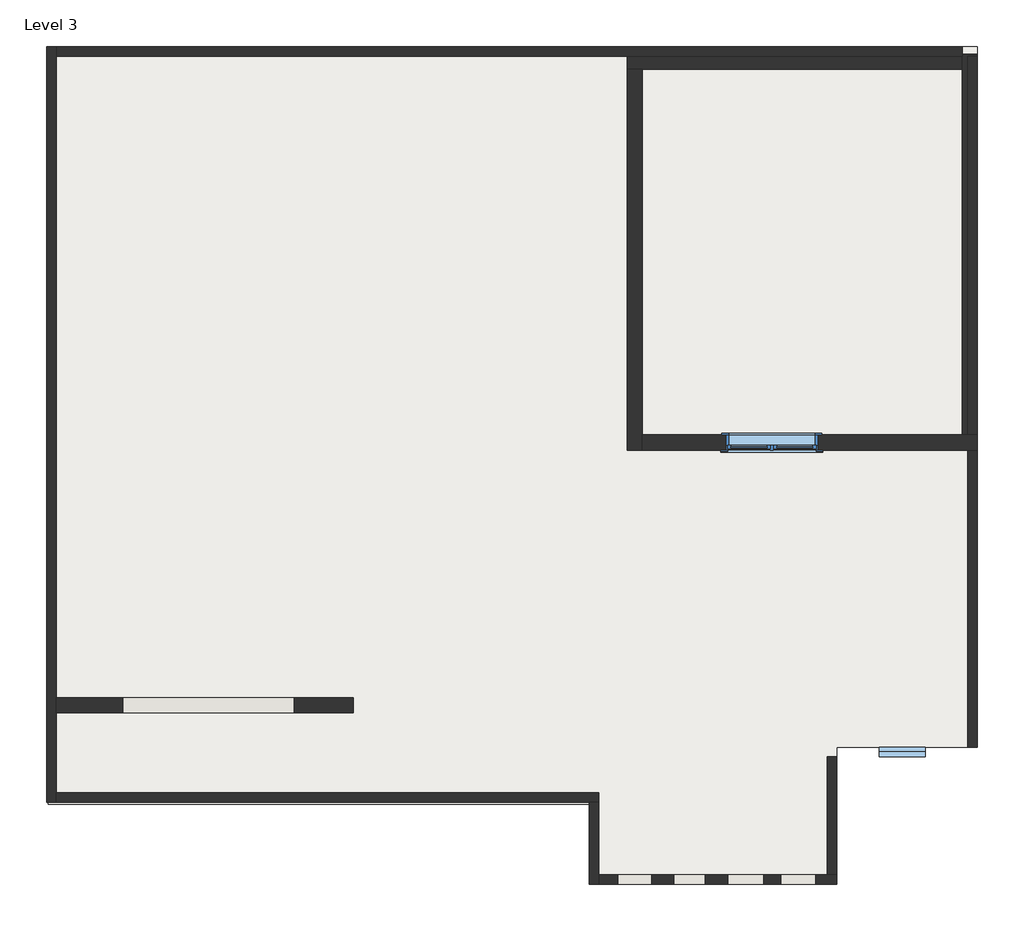
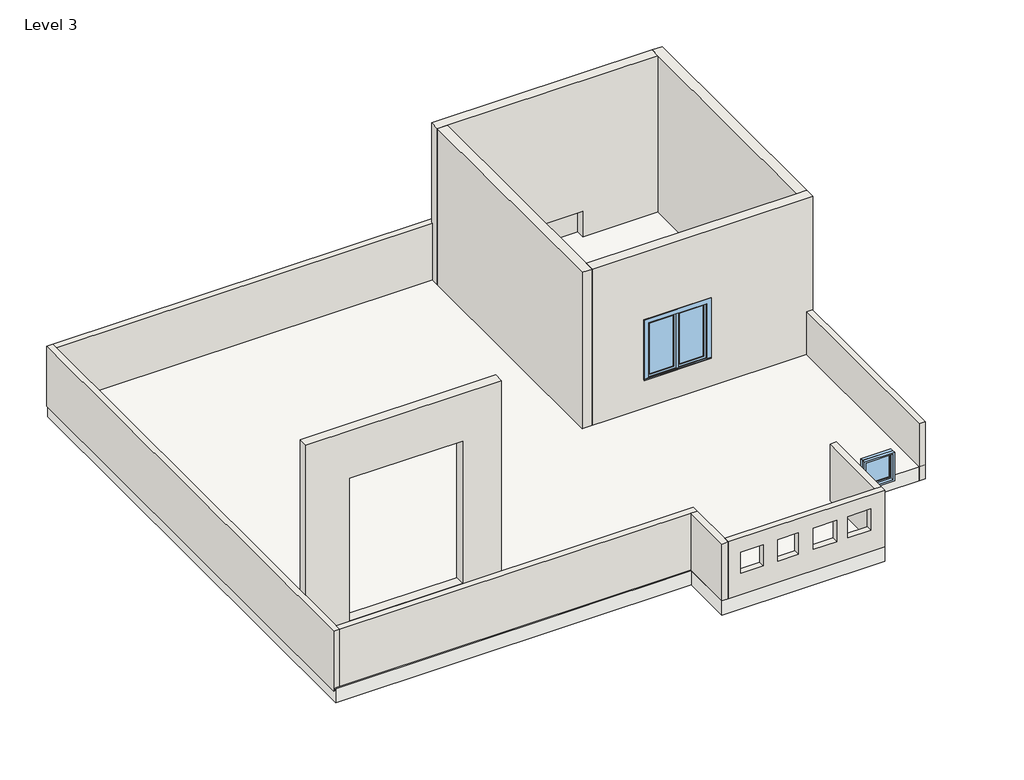
# One storey: 12 walls, 2 windows, 1 roof.
"""IFC4 building model written with IfcOpenShell, lengths in millimetres."""

from ifc_helpers import new_model, si_unit, frame, origin, place, context, project, spatial, polyline, outline, extrude, faceted_brep, transform, mapped, element, save
from components import window_0862ab64, window_d757e824

model = new_model("IFC4")

# Units and contexts
model_context = context("Model", 3, world=origin())
ifc_project = project(units=[si_unit("LENGTHUNIT", "METRE", prefix="MILLI")], contexts=[model_context])

# Site, building, storey
site = spatial("IfcSite", under=ifc_project)
building = spatial("IfcBuilding", under=site)
storey = spatial("IfcBuildingStorey", under=building, Name="Level 3", Elevation=7315.2)

# Roof
placement = place(None, origin())
element("IfcRoof", 1, ObjectType="Generic - 12\"", at=placement, inside=storey, context=model_context, shape_type="SweptSolid", body=[
    extrude(outline(polyline([(-15765.530251, 14053.673096), (-5249.930251, 14053.673096), (-3370.330251, 14053.673096), (-3370.330251, 4706.473096), (-5249.930251, 4706.473096), (-5249.930251, 2877.673096), (-8551.930251, 2877.673096), (-8551.930251, 3944.473096), (-15765.530251, 3944.473096), (-15765.530251, 14053.673096)])), frame((0.0, 0.0, 7315.2), z_axis=(0.0, 0.0, 1.0), x_axis=(1.0, 0.0, 0.0)), (0.0, 0.0, 1.0), 304.8),
])

# Walls
element("IfcWall", 2, ObjectType="Generic - 5\"", at=placement, inside=storey, context=model_context, shape_type="Brep", body=[
    faceted_brep([(-15790.930251, 14053.673096, 7553.9298874), (-15790.930251, 3969.873096, 7553.9298874), (-15790.930251, 3969.873096, 8839.2), (-15790.930251, 14053.673096, 8839.2), (-15663.930251, 14053.673096, 7553.9298874), (-15663.930251, 14053.673096, 8839.2), (-15663.930251, 13926.673096, 8839.2), (-15663.930251, 4096.873096, 8839.2), (-15663.930251, 3969.873096, 8839.2), (-15663.930251, 3969.873096, 7620.0), (-15663.930251, 3969.873096, 7553.9298874)], [[[0, 1, 2, 3]], [[4, 5, 6, 7, 8, 9, 10]], [[1, 0, 4, 10]], [[3, 2, 8, 7, 6, 5]], [[2, 1, 10, 9, 8]], [[0, 3, 5, 4]]]),
])
element("IfcWall", 3, ObjectType="Generic - 5\"", at=placement, inside=storey, context=model_context, shape_type="Brep", body=[
    faceted_brep([(-15663.930251, 3969.873096, 7620.0), (-8551.930251, 3969.873096, 7620.0), (-8424.930251, 3969.873096, 7620.0), (-8424.930251, 3969.873096, 8839.2), (-8551.930251, 3969.873096, 8839.2), (-15663.930251, 3969.873096, 8839.2), (-15663.930251, 4096.873096, 7620.0), (-15663.930251, 4096.873096, 8839.2), (-8424.930251, 4096.873096, 8839.2), (-8424.930251, 4096.873096, 7620.0)], [[[0, 1, 2, 3, 4, 5]], [[6, 7, 8, 9]], [[2, 1, 0, 6, 9]], [[5, 4, 3, 8, 7]], [[0, 5, 7, 6]], [[3, 2, 9, 8]]]),
])
element("IfcWall", 4, ObjectType="Generic - 5\"", at=placement, inside=storey, context=model_context, shape_type="Brep", body=[
    faceted_brep([(-8551.930251, 3969.873096, 7620.0), (-8551.930251, 2877.673096, 7620.0), (-8551.930251, 2877.673096, 8839.2), (-8551.930251, 3969.873096, 8839.2), (-8424.930251, 3969.873096, 7620.0), (-8424.930251, 3969.873096, 8839.2), (-8424.930251, 3004.673096, 8839.2), (-8424.930251, 2877.673096, 8839.2), (-8424.930251, 2877.673096, 7620.0), (-8424.930251, 3004.673096, 7620.0)], [[[0, 1, 2, 3]], [[4, 5, 6, 7, 8, 9]], [[1, 0, 4, 9, 8]], [[3, 2, 7, 6, 5]], [[0, 3, 5, 4]], [[2, 1, 8, 7]]]),
])
element("IfcWall", 5, ObjectType="Generic - 5\"", at=placement, inside=storey, context=model_context, shape_type="Brep", body=[
    faceted_brep([(-8424.930251, 2877.673096, 7620.0), (-5249.930251, 2877.673096, 7620.0), (-5249.930251, 2877.673096, 8839.2), (-8424.930251, 2877.673096, 8839.2), (-7713.730251, 2877.673096, 8534.4), (-7713.730251, 2877.673096, 8077.2), (-8170.930251, 2877.673096, 8077.2), (-8170.930251, 2877.673096, 8534.4), (-6999.8257201, 2877.673096, 8534.4), (-6999.8257201, 2877.673096, 8077.2), (-7421.8476525, 2877.673096, 8077.2), (-7421.8476525, 2877.673096, 8534.4), (-6222.21017, 2877.673096, 8534.4), (-6222.21017, 2877.673096, 8077.2), (-6702.8462596, 2877.673096, 8077.2), (-6702.8462596, 2877.673096, 8534.4), (-5529.330251, 2877.673096, 8534.4), (-5529.330251, 2877.673096, 8077.2), (-5995.5708893, 2877.673096, 8077.2), (-5995.5708893, 2877.673096, 8534.4), (-8424.930251, 3004.673096, 7620.0), (-8424.930251, 3004.673096, 8839.2), (-5376.930251, 3004.673096, 8839.2), (-5249.930251, 3004.673096, 8839.2), (-5249.930251, 3004.673096, 7620.0), (-7713.730251, 3004.673096, 8534.4), (-8170.930251, 3004.673096, 8534.4), (-8170.930251, 3004.673096, 8077.2), (-7713.730251, 3004.673096, 8077.2), (-6999.8257201, 3004.673096, 8534.4), (-7421.8476525, 3004.673096, 8534.4), (-7421.8476525, 3004.673096, 8077.2), (-6999.8257201, 3004.673096, 8077.2), (-6222.21017, 3004.673096, 8534.4), (-6702.8462596, 3004.673096, 8534.4), (-6702.8462596, 3004.673096, 8077.2), (-6222.21017, 3004.673096, 8077.2), (-5529.330251, 3004.673096, 8534.4), (-5995.5708893, 3004.673096, 8534.4), (-5995.5708893, 3004.673096, 8077.2), (-5529.330251, 3004.673096, 8077.2)], [[[0, 1, 2, 3], [4, 5, 6, 7], [8, 9, 10, 11], [12, 13, 14, 15], [16, 17, 18, 19]], [[20, 21, 22, 23, 24], [25, 26, 27, 28], [29, 30, 31, 32], [33, 34, 35, 36], [37, 38, 39, 40]], [[0, 3, 21, 20]], [[2, 1, 24, 23]], [[1, 0, 20, 24]], [[3, 2, 23, 22, 21]], [[5, 4, 25, 28]], [[6, 5, 28, 27]], [[7, 6, 27, 26]], [[4, 7, 26, 25]], [[9, 8, 29, 32]], [[10, 9, 32, 31]], [[11, 10, 31, 30]], [[8, 11, 30, 29]], [[13, 12, 33, 36]], [[14, 13, 36, 35]], [[15, 14, 35, 34]], [[12, 15, 34, 33]], [[17, 16, 37, 40]], [[18, 17, 40, 39]], [[19, 18, 39, 38]], [[16, 19, 38, 37]]]),
])
element("IfcWall", 6, ObjectType="Generic - 5\"", at=placement, inside=storey, context=model_context, shape_type="Brep", body=[
    faceted_brep([(-5249.930251, 3004.673096, 7315.2), (-5249.930251, 4579.473096, 7315.2), (-5249.930251, 4579.473096, 8839.2), (-5249.930251, 3004.673096, 8839.2), (-5249.930251, 3004.673096, 7620.0), (-5376.930251, 3004.673096, 7315.2), (-5376.930251, 3004.673096, 8839.2), (-5376.930251, 4579.473096, 8839.2), (-5376.930251, 4579.473096, 7315.2)], [[[0, 1, 2, 3, 4]], [[5, 6, 7, 8]], [[1, 0, 5, 8]], [[3, 2, 7, 6]], [[2, 1, 8, 7]], [[0, 4, 3, 6, 5]]]),
])
element("IfcWall", 7, ObjectType="Generic - 5\"", at=placement, inside=storey, context=model_context, shape_type="Brep", body=[
    faceted_brep([(-15663.930251, 13926.673096, 7315.2), (-3573.530251, 13926.673096, 7315.2), (-3573.530251, 13926.673096, 8839.2), (-15663.930251, 13926.673096, 8839.2), (-15663.930251, 14053.673096, 7315.2), (-15663.930251, 14053.673096, 7553.9298874), (-15663.930251, 14053.673096, 8839.2), (-3573.530251, 14053.673096, 8839.2), (-3573.530251, 14053.673096, 7315.2), (-3573.530251, 13952.073096, 7315.2)], [[[0, 1, 2, 3]], [[4, 5, 6, 7, 8]], [[1, 0, 4, 8, 9]], [[3, 2, 7, 6]], [[0, 3, 6, 5, 4]], [[1, 9, 8, 7, 2]]]),
])
element("IfcWall", 8, ObjectType="Generic - 5\"", at=placement, inside=storey, context=model_context, shape_type="SweptSolid", body=[
    extrude(outline(polyline([(-3497.330251, 4706.473096), (-3497.330251, 13926.673096), (-3370.330251, 13926.673096), (-3370.330251, 4706.473096), (-3497.330251, 4706.473096)])), frame((0.0, 0.0, 7315.2), z_axis=(0.0, 0.0, 1.0), x_axis=(1.0, 0.0, 0.0)), (0.0, 0.0, 1.0), 1219.2),
])
element("IfcWall", 9, ObjectType="Generic - 8\"", at=placement, inside=storey, context=model_context, shape_type="Brep", body=[
    faceted_brep([(-8043.930251, 13748.873096, 10972.8), (-8043.930251, 13748.873096, 7315.2), (-7840.730251, 13748.873096, 7315.2), (-6316.730251, 13748.873096, 7315.2), (-6316.730251, 13748.873096, 8168.8474745), (-5097.530251, 13748.873096, 8168.8474745), (-5097.530251, 13748.873096, 7315.2), (-3573.530251, 13748.873096, 7315.2), (-3573.530251, 13748.873096, 10972.8), (-7840.730251, 13748.873096, 10972.8), (-8043.930251, 13952.073096, 7315.2), (-8043.930251, 13952.073096, 10972.8), (-3573.530251, 13952.073096, 10972.8), (-3573.530251, 13952.073096, 7315.2), (-5097.530251, 13952.073096, 7315.2), (-5097.530251, 13952.073096, 8168.8474745), (-6316.730251, 13952.073096, 8168.8474745), (-6316.730251, 13952.073096, 7315.2)], [[[0, 1, 2, 3, 4, 5, 6, 7, 8, 9]], [[10, 11, 12, 13, 14, 15, 16, 17]], [[1, 10, 17, 3, 2]], [[13, 7, 6, 14]], [[1, 0, 11, 10]], [[0, 9, 8, 12, 11]], [[7, 13, 12, 8]], [[16, 4, 3, 17]], [[5, 15, 14, 6]], [[4, 16, 15, 5]]]),
])
element("IfcWall", 10, ObjectType="Generic - 8\"", at=placement, inside=storey, context=model_context, shape_type="Brep", body=[
    faceted_brep([(-7840.730251, 8668.873096, 7315.2), (-7840.730251, 8872.073096, 7315.2), (-7840.730251, 13748.873096, 7315.2), (-7840.730251, 13748.873096, 10972.8), (-7840.730251, 8872.073096, 10972.8), (-7840.730251, 8668.873096, 10972.8), (-8043.930251, 8668.873096, 7315.2), (-8043.930251, 8668.873096, 10972.8), (-8043.930251, 13748.873096, 10972.8), (-8043.930251, 13748.873096, 7315.2)], [[[0, 1, 2, 3, 4, 5]], [[6, 7, 8, 9]], [[2, 1, 0, 6, 9]], [[0, 5, 7, 6]], [[3, 2, 9, 8]], [[5, 4, 3, 8, 7]]]),
])
element("IfcWall", 11, ObjectType="Generic - 8\"", at=placement, inside=storey, context=model_context, shape_type="Brep", body=[
    faceted_brep([(-3370.330251, 8872.073096, 7315.2), (-3573.530251, 8872.073096, 7315.2), (-7840.730251, 8872.073096, 7315.2), (-7840.730251, 8872.073096, 10972.8), (-3573.530251, 8872.073096, 10972.8), (-3370.330251, 8872.073096, 10972.8), (-6723.130251, 8872.073096, 9448.8), (-6723.130251, 8872.073096, 8229.6), (-5503.930251, 8872.073096, 8229.6), (-5503.930251, 8872.073096, 9448.8), (-3370.330251, 8668.873096, 7315.2), (-3370.330251, 8668.873096, 10972.8), (-7840.730251, 8668.873096, 10972.8), (-7840.730251, 8668.873096, 7315.2), (-6723.130251, 8668.873096, 9448.8), (-5503.930251, 8668.873096, 9448.8), (-5503.930251, 8668.873096, 8229.6), (-6723.130251, 8668.873096, 8229.6)], [[[0, 1, 2, 3, 4, 5], [6, 7, 8, 9]], [[10, 11, 12, 13], [14, 15, 16, 17]], [[2, 1, 0, 10, 13]], [[0, 5, 11, 10]], [[3, 2, 13, 12]], [[5, 4, 3, 12, 11]], [[7, 6, 14, 17]], [[8, 7, 17, 16]], [[9, 8, 16, 15]], [[6, 9, 15, 14]]]),
])
element("IfcWall", 12, ObjectType="Generic - 8\"", at=placement, inside=storey, context=model_context, shape_type="Brep", body=[
    faceted_brep([(-3573.530251, 13952.073096, 7315.2), (-3573.530251, 13926.673096, 7315.2), (-3573.530251, 13748.873096, 7315.2), (-3573.530251, 8872.073096, 7315.2), (-3573.530251, 8872.073096, 10972.8), (-3573.530251, 13748.873096, 10972.8), (-3573.530251, 13952.073096, 10972.8), (-3370.330251, 13952.073096, 7315.2), (-3370.330251, 13952.073096, 10972.8), (-3370.330251, 8872.073096, 10972.8), (-3370.330251, 8872.073096, 7315.2)], [[[0, 1, 2, 3, 4, 5, 6]], [[7, 8, 9, 10]], [[3, 2, 1, 0, 7, 10]], [[0, 6, 8, 7]], [[4, 3, 10, 9]], [[6, 5, 4, 9, 8]]]),
])
element("IfcWall", 13, ObjectType="Generic - 8\"", at=placement, inside=storey, context=model_context, shape_type="SweptSolid", body=[
    extrude(outline(polyline([(7315.2, -11701.530251), (12060.2211965, -11701.530251), (12060.2211965, -15663.930251), (7315.2, -15663.930251), (7315.2, -11701.530251)]), holes=[polyline([(11036.4557736, -12487.9209013), (7988.4557736, -12487.9209013), (7988.4557736, -14773.9209013), (11036.4557736, -14773.9209013), (11036.4557736, -12487.9209013)])]), frame((0.0, 5163.673096, 0.0), z_axis=(0.0, 1.0, 0.0), x_axis=(0.0, 0.0, 1.0)), (0.0, 0.0, 1.0), 203.2),
])

# Windows
window_shape = window_0862ab64(model_context)
element("IfcWindow", 14, ObjectType="Casement Dbl with Trim.0001 : 48\" x 48\"", at=placement, inside=storey, context=model_context, shape_type="MappedRepresentation", body=[
    mapped(window_shape, transform((-6113.530251, 8789.523096, 7315.2), x_axis=(-1.0, 0.0, 0.0), y_axis=(0.0, -1.0, 0.0), z_axis=(0.0, 0.0, 1.0))),
])
window_2_shape = window_d757e824(model_context)
element("IfcWindow", 15, ObjectType="Fixed : 24\" x 24\"", at=placement, inside=storey, context=model_context, shape_type="MappedRepresentation", body=[
    mapped(window_2_shape, transform((-4335.530251, 4642.973096, 6679.7905952), x_axis=(1.0, 0.0, 0.0), y_axis=(0.0, 1.0, 0.0), z_axis=(0.0, 0.0, 1.0))),
])

save(model, "model.ifc")

# Revit data of these elements
# Type "Generic - 12\""
#   Assembly Code = "B1020"
#   Layers, outside or top first: 1' - 0" no material (function 1)
# Type "Generic - 5\""
#   Assembly Code = "B2010"
#   Layers, outside or top first: 0' - 5" no material (function 1)
# Type "Generic - 8\""
#   Assembly Code = "B2010"
#   Layers, outside or top first: 0' - 8" no material (function 1)
# Type "Casement Dbl with Trim.0001 : 48\" x 48\""
#   Type Mark = "10"
#   Construction Type Id = "GSP4R"
#   Assembly Code = "B2020100"
#   Analytic Construction = "1/8 in Pilkington single glazing"
#   Visual Light Transmittance = 0.9
#   Solar Heat Gain Coefficient = 0.78
#   Heat Transfer Coefficient (U) = 0.6496 BTU/(h·ft²·°F)
#   Height = 4' - 0"
#   Default Sill Height = 3' - 0"
#   Trim Projection - Ext. = 0' - 0 1/2"
#   Trim Projection - Int. = 0' - 0 3/4"
#   Trim Width - Exterior = 0' - 3 1/2"
#   Trim Width - Interior = 0' - 3 1/2"
#   Width = 4' - 0"
#   Window Inset = 0' - 0 3/4"
#   Define Thermal Properties by = 1
#   Glass Pane Material = Glass
#   Sash Material = Sash
#   Trim Exterior Material = Trim
#   Trim Interior Material = Trim
#   Wall Closure = (empty or 0)
# Type "Fixed : 24\" x 24\""
#   Type Mark = "3"
#   Construction Type Id = "GSP4R"
#   Assembly Code = "B2020100"
#   Analytic Construction = "1/8 in Pilkington single glazing"
#   Visual Light Transmittance = 0.9
#   Solar Heat Gain Coefficient = 0.78
#   Heat Transfer Coefficient (U) = 0.6496 BTU/(h·ft²·°F)
#   Height = 2' - 0"
#   Default Sill Height = 3' - 0"
#   Width = 2' - 0"
#   Window Inset = 0' - 0 3/4"
#   Define Thermal Properties by = 1
#   Glass Pane Material = Glass
#   Sash Material = Sash
#   Wall Closure = (empty or 0)
# Element 1 (IfcRoof, "Generic - 12\"")
#   built-in parameter 1001705 = 25 (stored number, unit not read)
#   built-in parameter 1001710 = 33615
#   Phase Created = New Construction
#   Materials on its faces: "Default Roof"
# Element 2 (IfcWall, "Generic - 5\"")
#   built-in parameter 1001111 = 0' - 9.39881"
#   Top Offset = -7' - 0"
#   Base Offset = 0' - 9.39881"
#   wall height = 4' - 2.60119"
#   Phase Created = New Construction
#   Base Constraint = Level 3
#   Top Constraint = Level 4
#   Materials on its faces: "Default Wall"
# Elements 3, 4, 5 (IfcWall, "Generic - 5\"")
#   built-in parameter 1001111 = 1' - 0"
#   Top Offset = -7' - 0"
#   Base Offset = 1' - 0"
#   wall height = 4' - 0"
#   Phase Created = New Construction
#   Base Constraint = Level 3
#   Top Constraint = Level 4
#   Materials on its faces: "Default Wall"
# Elements 6, 7 (IfcWall, "Generic - 5\"")
#   Top Offset = -7' - 0"
#   Base Offset = 0' - 0"
#   wall height = 5' - 0"
#   Phase Created = New Construction
#   Base Constraint = Level 3
#   Top Constraint = Level 4
#   Materials on its faces: "Default Wall"
# Element 8 (IfcWall, "Generic - 5\"")
#   Top Offset = -8' - 0"
#   Base Offset = 0' - 0"
#   wall height = 4' - 0"
#   Phase Created = New Construction
#   Base Constraint = Level 3
#   Top Constraint = Level 4
#   Materials on its faces: "Default Wall"
# Elements 9, 10, 11, 12 (IfcWall, "Generic - 8\"")
#   Top Offset = 0' - 0"
#   Base Offset = 0' - 0"
#   Unconnected Height = 12' - 0"
#   wall height = 12' - 0"
#   Phase Created = New Construction
#   Base Constraint = Level 3
#   Materials on its faces: "Default Wall"
# Element 13 (IfcWall, "Generic - 8\"")
#   Top Offset = 0' - 0"
#   Base Offset = 0' - 0"
#   Unconnected Height = 15' - 6.81186"
#   wall height = 15' - 6.81186"
#   Phase Created = New Construction
#   Base Constraint = Level 3
#   Materials on its faces: "Default Wall"
# Element 14 (IfcWindow, "Casement Dbl with Trim.0001 : 48\" x 48\"")
#   Mark = "4"
#   Phase Created = New Construction
#   Materials on its faces: "Sash", "Trim", "Glass"
# Element 15 (IfcWindow, "Fixed : 24\" x 24\"")
#   Mark = "1"
#   Phase Created = New Construction
#   Materials on its faces: "Sash", "Glass"
# Materials
#   "Glass": class "Glass", colour RGB 0 128 192, transparency 0.75, Description = "Soda Lime Glass", Cost = 0
#   "Sash": class "Wood", colour RGB 224 178 126, transparency 0
#   "Trim": class "Wood", colour RGB 224 178 126, transparency 0
#   "Default Roof": colour RGB 88 101 114, transparency 0
#   "Default Wall": colour RGB 128 128 128, transparency 0
